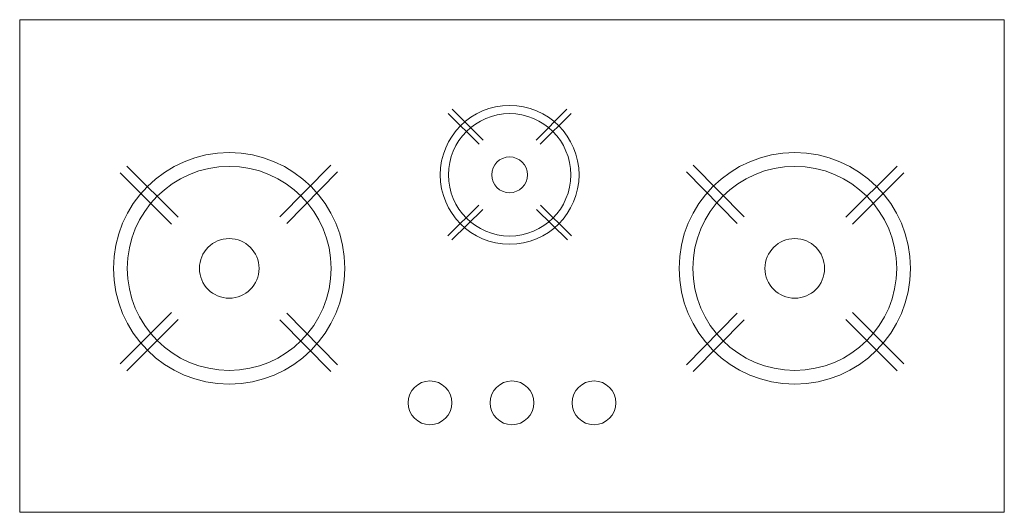
# Model space of a CAD drawing. Units: inches. Extents: x -26 to 13070, y -956 to 6917.
# Tile 12 of 13: x 6307 to 7207, y 6467 to 6917. Entities that reach past the tile are written whole.
import ezdxf

# ---------------------------------------------------------------- set-up
doc = ezdxf.new("R2010")
doc.units = ezdxf.units.IN
doc.header["$MEASUREMENT"] = 0
doc.layers.add('A-EQPM', color=8, linetype='Continuous', lineweight=18)

msp = doc.modelspace()

# ---------------------------------------------------------------- linework, layer by layer
at = {"layer": 'A-EQPM'}
for p, q in [((7207.357, 6917.459), (6307.357, 6917.459)), ((6307.357, 6917.459), (6307.357, 6467.459)), ((7207.357, 6467.459), (7207.357, 6917.459)), ((6727.196, 6803.739), (6699.085, 6831.851)), ((6730.93, 6807.473), (6702.818, 6835.585)), ((6779.454, 6807.473), (6807.565, 6835.585)), ((6783.187, 6803.739), (6811.299, 6831.851)), ((6446, 6730.73), (6399.148, 6777.583)), ((6452.223, 6736.953), (6405.37, 6783.805)), ((6545.174, 6737.317), (6591.659, 6784.535)), ((6551.445, 6731.143), (6597.93, 6778.361)), ((6963.27, 6731.143), (6916.785, 6778.361)), ((6969.541, 6737.317), (6923.056, 6784.535)), ((7062.492, 6736.953), (7109.345, 6783.805)), ((7068.715, 6730.73), (7115.567, 6777.583)), ((6726.978, 6747.969), (6698.647, 6720.078)), ((6730.682, 6744.206), (6702.351, 6716.315)), ((6779.702, 6744.206), (6808.032, 6716.315)), ((6783.406, 6747.969), (6811.737, 6720.078)), ((6446, 6649.857), (6399.148, 6603.004)), ((6452.223, 6643.634), (6405.37, 6596.782)), ((6545.174, 6643.27), (6591.659, 6596.052)), ((6551.445, 6649.444), (6597.93, 6602.226)), ((6963.27, 6649.444), (6916.785, 6602.226)), ((6969.541, 6643.27), (6923.056, 6596.052)), ((7062.492, 6643.634), (7109.345, 6596.782)), ((7068.715, 6649.857), (7115.567, 6603.004)), ((6307.357, 6467.459), (7207.357, 6467.459))]:
    msp.add_line(p, q, dxfattribs=at)
for centre, radius in [((6755.192, 6775.744), 63.433), ((6755.192, 6775.744), 55.902), ((6498.882, 6690.293), 105.722), ((7015.833, 6690.293), 105.722), ((6755.192, 6775.744), 16.356), ((6498.882, 6690.293), 93.171), ((7015.833, 6690.293), 93.171), ((6498.882, 6690.293), 27.26), ((7015.833, 6690.293), 27.26), ((6682.357, 6567.459), 20), ((6757.357, 6567.459), 20), ((6832.357, 6567.459), 20)]:
    msp.add_circle(centre, radius, dxfattribs=at)

doc.saveas('drawing.dxf')
